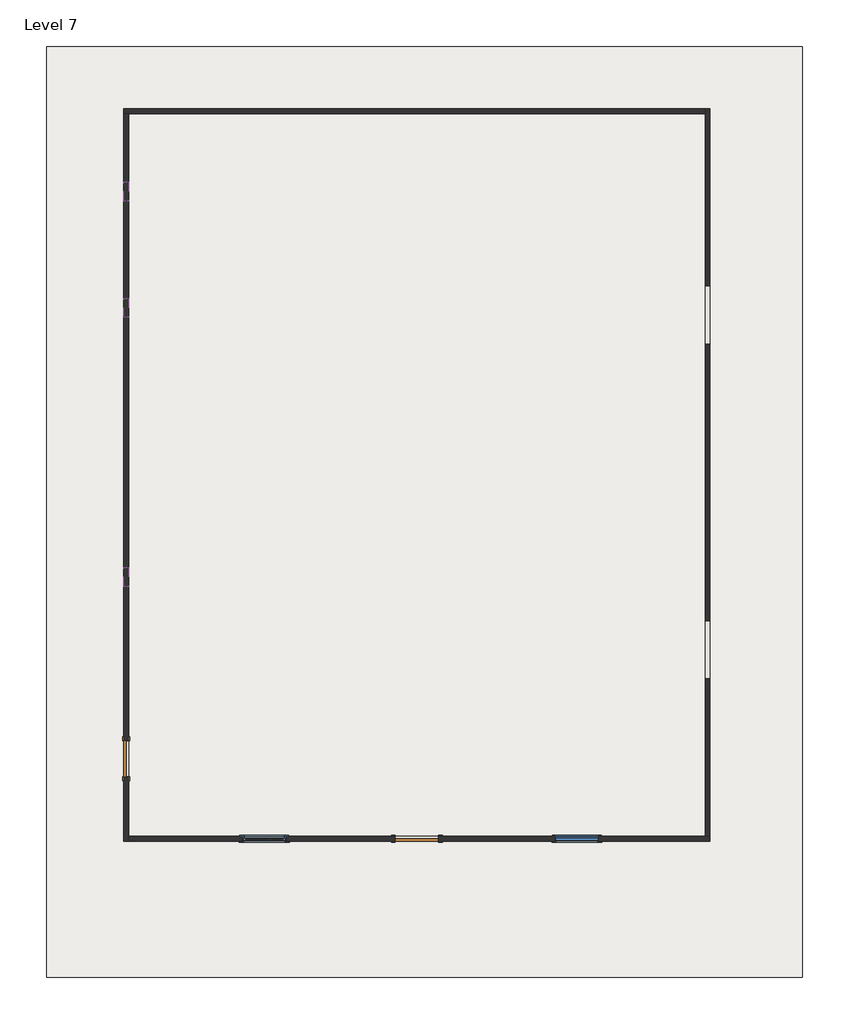
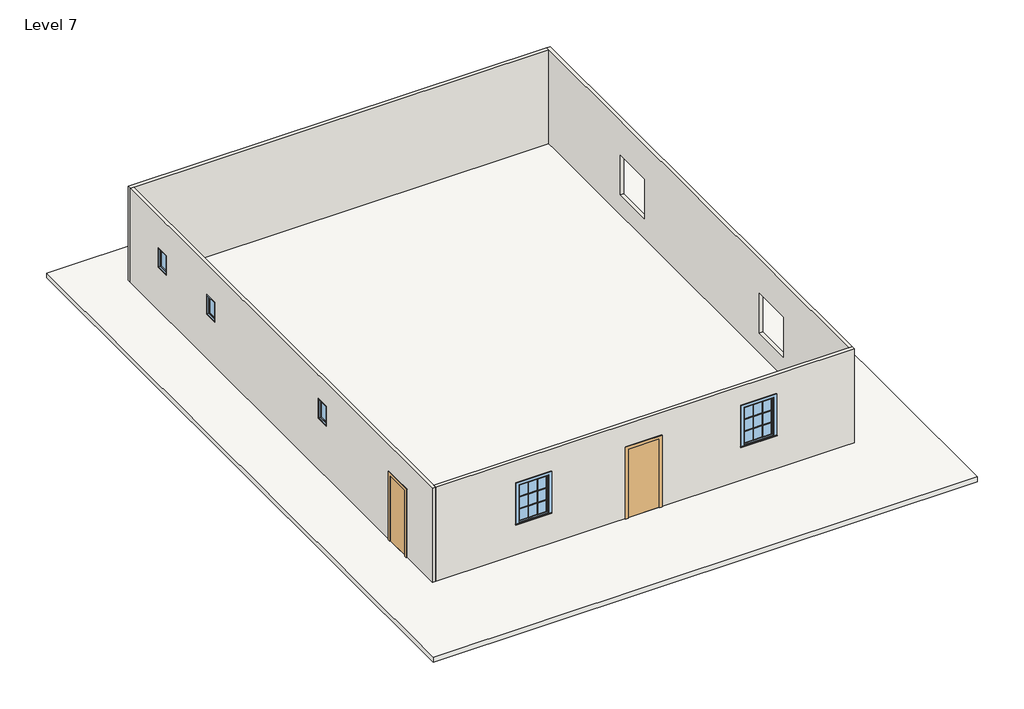
# One storey, incomplete: 5 windows, 4 walls, 2 doors, 1 roof.
"""IFC4 building model written with IfcOpenShell, lengths in millimetres."""

from ifc_helpers import new_model, si_unit, frame, origin, place, context, project, spatial, polyline, outline, extrude, faceted_brep, transform, mapped, element, save
from components import door_29583826, door_048588e9, window_ad8769eb, window_a112695e

model = new_model("IFC4")

# Units and contexts
model_context = context("Model", 3, world=origin())
ifc_project = project(units=[si_unit("LENGTHUNIT", "METRE", prefix="MILLI")], contexts=[model_context])

# Site, building, storey
site = spatial("IfcSite", under=ifc_project)
building = spatial("IfcBuilding", under=site)
storey = spatial("IfcBuildingStorey", under=building, Name="Level 7", Elevation=9601.2)

# Doors
placement = place(None, origin())
door_shape = door_29583826(model_context)
element("IfcDoor", 1, ObjectType="Single-Flush : 30\" x 80\"", at=placement, inside=storey, context=model_context, shape_type="MappedRepresentation", body=[
    mapped(door_shape, transform((1744.5168112, -314.4718204, 9753.6), x_axis=(0.0, 1.0, 0.0), y_axis=(-1.0, 0.0, 0.0), z_axis=(0.0, 0.0, 1.0))),
])
door_2_shape = door_048588e9(model_context)
element("IfcDoor", 2, ObjectType="Single-Flush : 36\" x 84\"", at=placement, inside=storey, context=model_context, shape_type="MappedRepresentation", body=[
    mapped(door_2_shape, transform((7840.5168112, -1990.8718204, 9753.6), x_axis=(-1.0, 0.0, 0.0), y_axis=(0.0, -1.0, 0.0), z_axis=(0.0, 0.0, 1.0))),
])

# Roof
element("IfcRoof", 3, ObjectType="6", at=placement, inside=storey, context=model_context, shape_type="SweptSolid", body=[
    extrude(outline(polyline([(74.1689082, 14608.7600271), (15923.7689082, 14608.7600271), (15923.7689082, -4898.4399729), (74.1689082, -4898.4399729), (74.1689082, 14608.7600271)])), frame((0.0, 0.0, 9601.2), z_axis=(0.0, 0.0, 1.0), x_axis=(1.0, 0.0, 0.0)), (0.0, 0.0, 1.0), 152.4),
])

# Walls
element("IfcWall", 4, ObjectType="Generic - 4\" Brick", at=placement, inside=storey, context=model_context, shape_type="Brep", body=[
    faceted_brep([(1693.7168112, 13198.3281796, 9601.2), (1795.3168112, 13198.3281796, 9601.2), (13885.7168112, 13198.3281796, 9601.2), (13885.7168112, 13198.3281796, 12649.2), (1795.3168112, 13198.3281796, 12649.2), (1693.7168112, 13198.3281796, 12649.2), (1693.7168112, 13299.9281796, 9601.2), (1693.7168112, 13299.9281796, 12649.2), (13885.7168112, 13299.9281796, 12649.2), (13885.7168112, 13299.9281796, 9601.2)], [[[0, 1, 2, 3, 4, 5]], [[6, 7, 8, 9]], [[2, 1, 0, 6, 9]], [[0, 5, 7, 6]], [[3, 2, 9, 8]], [[5, 4, 3, 8, 7]]]),
])
element("IfcWall", 5, ObjectType="Generic - 4\" Brick", at=placement, inside=storey, context=model_context, shape_type="Brep", body=[
    faceted_brep([(1795.3168112, -2041.6718204, 9601.2), (1795.3168112, -1940.0718204, 9601.2), (1795.3168112, 13198.3281796, 9601.2), (1795.3168112, 13198.3281796, 12649.2), (1795.3168112, -1940.0718204, 12649.2), (1795.3168112, -2041.6718204, 12649.2), (1795.3168112, -695.4718204, 9753.6), (1795.3168112, -695.4718204, 11785.6), (1795.3168112, 66.5281796, 11785.6), (1795.3168112, 66.5281796, 9753.6), (1795.3168112, 11369.5281796, 11689.2182753), (1795.3168112, 11775.9281796, 11689.2182753), (1795.3168112, 11775.9281796, 11079.6182753), (1795.3168112, 11369.5281796, 11079.6182753), (1795.3168112, 8931.1281796, 11725.7539428), (1795.3168112, 9337.5281796, 11725.7539428), (1795.3168112, 9337.5281796, 11116.1539428), (1795.3168112, 8931.1281796, 11116.1539428), (1795.3168112, 3292.3281796, 11939.4851545), (1795.3168112, 3698.7281796, 11939.4851545), (1795.3168112, 3698.7281796, 11329.8851545), (1795.3168112, 3292.3281796, 11329.8851545), (1693.7168112, -2041.6718204, 9601.2), (1693.7168112, -2041.6718204, 12649.2), (1693.7168112, 13198.3281796, 12649.2), (1693.7168112, 13198.3281796, 9601.2), (1693.7168112, -695.4718204, 9753.6), (1693.7168112, 66.5281796, 9753.6), (1693.7168112, 66.5281796, 11785.6), (1693.7168112, -695.4718204, 11785.6), (1693.7168112, 11369.5281796, 11689.2182753), (1693.7168112, 11369.5281796, 11079.6182753), (1693.7168112, 11775.9281796, 11079.6182753), (1693.7168112, 11775.9281796, 11689.2182753), (1693.7168112, 8931.1281796, 11725.7539428), (1693.7168112, 8931.1281796, 11116.1539428), (1693.7168112, 9337.5281796, 11116.1539428), (1693.7168112, 9337.5281796, 11725.7539428), (1693.7168112, 3292.3281796, 11939.4851545), (1693.7168112, 3292.3281796, 11329.8851545), (1693.7168112, 3698.7281796, 11329.8851545), (1693.7168112, 3698.7281796, 11939.4851545)], [[[0, 1, 2, 3, 4, 5], [6, 7, 8, 9], [10, 11, 12, 13], [14, 15, 16, 17], [18, 19, 20, 21]], [[22, 23, 24, 25], [26, 27, 28, 29], [30, 31, 32, 33], [34, 35, 36, 37], [38, 39, 40, 41]], [[2, 1, 0, 22, 25]], [[0, 5, 23, 22]], [[3, 2, 25, 24]], [[5, 4, 3, 24, 23]], [[27, 26, 6, 9]], [[28, 27, 9, 8]], [[29, 28, 8, 7]], [[26, 29, 7, 6]], [[31, 30, 10, 13]], [[32, 31, 13, 12]], [[33, 32, 12, 11]], [[30, 33, 11, 10]], [[35, 34, 14, 17]], [[36, 35, 17, 16]], [[37, 36, 16, 15]], [[34, 37, 15, 14]], [[39, 38, 18, 21]], [[40, 39, 21, 20]], [[41, 40, 20, 19]], [[38, 41, 19, 18]]]),
])
element("IfcWall", 6, ObjectType="Generic - 4\" Brick", at=placement, inside=storey, context=model_context, shape_type="Brep", body=[
    faceted_brep([(13987.3168112, -1940.0718204, 9601.2), (13885.7168112, -1940.0718204, 9601.2), (1795.3168112, -1940.0718204, 9601.2), (1795.3168112, -1940.0718204, 12649.2), (13885.7168112, -1940.0718204, 12649.2), (13987.3168112, -1940.0718204, 12649.2), (8297.7168112, -1940.0718204, 9753.6), (8297.7168112, -1940.0718204, 11887.2), (7383.3168112, -1940.0718204, 11887.2), (7383.3168112, -1940.0718204, 9753.6), (4182.9168112, -1940.0718204, 11907.6881646), (4182.9168112, -1940.0718204, 10688.4881646), (5097.3168112, -1940.0718204, 10688.4881646), (5097.3168112, -1940.0718204, 11907.6881646), (10736.1168112, -1940.0718204, 11999.2796438), (10736.1168112, -1940.0718204, 10780.0796438), (11650.5168112, -1940.0718204, 10780.0796438), (11650.5168112, -1940.0718204, 11999.2796438), (13987.3168112, -2041.6718204, 9601.2), (13987.3168112, -2041.6718204, 12649.2), (1795.3168112, -2041.6718204, 12649.2), (1795.3168112, -2041.6718204, 9601.2), (8297.7168112, -2041.6718204, 9753.6), (7383.3168112, -2041.6718204, 9753.6), (7383.3168112, -2041.6718204, 11887.2), (8297.7168112, -2041.6718204, 11887.2), (4182.9168112, -2041.6718204, 11907.6881646), (5097.3168112, -2041.6718204, 11907.6881646), (5097.3168112, -2041.6718204, 10688.4881646), (4182.9168112, -2041.6718204, 10688.4881646), (10736.1168112, -2041.6718204, 11999.2796438), (11650.5168112, -2041.6718204, 11999.2796438), (11650.5168112, -2041.6718204, 10780.0796438), (10736.1168112, -2041.6718204, 10780.0796438)], [[[0, 1, 2, 3, 4, 5], [6, 7, 8, 9], [10, 11, 12, 13], [14, 15, 16, 17]], [[18, 19, 20, 21], [22, 23, 24, 25], [26, 27, 28, 29], [30, 31, 32, 33]], [[2, 1, 0, 18, 21]], [[0, 5, 19, 18]], [[3, 2, 21, 20]], [[5, 4, 3, 20, 19]], [[23, 22, 6, 9]], [[24, 23, 9, 8]], [[25, 24, 8, 7]], [[22, 25, 7, 6]], [[11, 10, 26, 29]], [[12, 11, 29, 28]], [[13, 12, 28, 27]], [[10, 13, 27, 26]], [[15, 14, 30, 33]], [[16, 15, 33, 32]], [[17, 16, 32, 31]], [[14, 17, 31, 30]]]),
])
element("IfcWall", 7, ObjectType="Generic - 4\" Brick", at=placement, inside=storey, context=model_context, shape_type="Brep", body=[
    faceted_brep([(13885.7168112, 13299.9281796, 9601.2), (13885.7168112, 13198.3281796, 9601.2), (13885.7168112, -1940.0718204, 9601.2), (13885.7168112, -1940.0718204, 12649.2), (13885.7168112, 13198.3281796, 12649.2), (13885.7168112, 13299.9281796, 12649.2), (13885.7168112, 1361.9281796, 11582.4), (13885.7168112, 1361.9281796, 10363.2), (13885.7168112, 2581.1281796, 10363.2), (13885.7168112, 2581.1281796, 11582.4), (13885.7168112, 8372.3281796, 11582.4), (13885.7168112, 8372.3281796, 10363.2), (13885.7168112, 9591.5281796, 10363.2), (13885.7168112, 9591.5281796, 11582.4), (13987.3168112, 13299.9281796, 9601.2), (13987.3168112, 13299.9281796, 12649.2), (13987.3168112, -1940.0718204, 12649.2), (13987.3168112, -1940.0718204, 9601.2), (13987.3168112, 1361.9281796, 11582.4), (13987.3168112, 2581.1281796, 11582.4), (13987.3168112, 2581.1281796, 10363.2), (13987.3168112, 1361.9281796, 10363.2), (13987.3168112, 8372.3281796, 11582.4), (13987.3168112, 9591.5281796, 11582.4), (13987.3168112, 9591.5281796, 10363.2), (13987.3168112, 8372.3281796, 10363.2)], [[[0, 1, 2, 3, 4, 5], [6, 7, 8, 9], [10, 11, 12, 13]], [[14, 15, 16, 17], [18, 19, 20, 21], [22, 23, 24, 25]], [[2, 1, 0, 14, 17]], [[0, 5, 15, 14]], [[3, 2, 17, 16]], [[5, 4, 3, 16, 15]], [[7, 6, 18, 21]], [[8, 7, 21, 20]], [[9, 8, 20, 19]], [[6, 9, 19, 18]], [[11, 10, 22, 25]], [[12, 11, 25, 24]], [[13, 12, 24, 23]], [[10, 13, 23, 22]]]),
])

# Windows
window_shape = window_ad8769eb(model_context)
element("IfcWindow", 8, ObjectType="Casement 3x3 with Trim : 36\" x 48\"", at=placement, inside=storey, context=model_context, shape_type="MappedRepresentation", body=[
    mapped(window_shape, transform((4640.1168112, -1990.8718204, 9774.0881646), x_axis=(-1.0, 0.0, 0.0), y_axis=(0.0, -1.0, 0.0), z_axis=(0.0, 0.0, 1.0))),
])
element("IfcWindow", 9, ObjectType="Casement 3x3 with Trim : 36\" x 48\"", at=placement, inside=storey, context=model_context, shape_type="MappedRepresentation", body=[
    mapped(window_shape, transform((11193.3168112, -1990.8718204, 9865.6796438), x_axis=(-1.0, 0.0, 0.0), y_axis=(0.0, -1.0, 0.0), z_axis=(0.0, 0.0, 1.0))),
])
window_2_shape = window_a112695e(model_context)
element("IfcWindow", 10, ObjectType="Fixed : 16\" x 24\"", at=placement, inside=storey, context=model_context, shape_type="MappedRepresentation", body=[
    mapped(window_2_shape, transform((1744.5168112, 11534.6281796, 10165.2182753), x_axis=(0.0, -1.0, 0.0), y_axis=(1.0, 0.0, 0.0), z_axis=(0.0, 0.0, 1.0))),
])
element("IfcWindow", 11, ObjectType="Fixed : 16\" x 24\"", at=placement, inside=storey, context=model_context, shape_type="MappedRepresentation", body=[
    mapped(window_2_shape, transform((1744.5168112, 9096.2281796, 10201.7539428), x_axis=(0.0, -1.0, 0.0), y_axis=(1.0, 0.0, 0.0), z_axis=(0.0, 0.0, 1.0))),
])
element("IfcWindow", 12, ObjectType="Fixed : 16\" x 24\"", at=placement, inside=storey, context=model_context, shape_type="MappedRepresentation", body=[
    mapped(window_2_shape, transform((1744.5168112, 3457.4281796, 10415.4851545), x_axis=(0.0, -1.0, 0.0), y_axis=(1.0, 0.0, 0.0), z_axis=(0.0, 0.0, 1.0))),
])

save(model, "model.ifc")

# Revit data of these elements
# Type "Single-Flush : 30\" x 80\""
#   Type Mark = "5"
#   Construction Type Id = "MDOOR"
#   Assembly Code = "C1020"
#   Analytic Construction = "Metal"
#   Thickness = 0' - 2"
#   Heat Transfer Coefficient (U) = 0.651978 BTU/(h·ft²·°F)
#   Height = 6' - 8"
#   Trim Projection Ext = 0' - 1"
#   Trim Projection Int = 0' - 1"
#   Trim Width = 0' - 3"
#   Width = 2' - 6"
#   Define Thermal Properties by = 1
#   Door Material = Door - Panel
#   Frame Material = Door - Frame
#   Visual Light Transmittance = 0
#   Solar Heat Gain Coefficient = 0
#   Function = (empty or 0)
#   Wall Closure = (empty or 0)
# Type "Single-Flush : 36\" x 84\""
#   Type Mark = "1"
#   Construction Type Id = "MDOOR"
#   Assembly Code = "C1020"
#   Analytic Construction = "Metal"
#   Thickness = 0' - 2"
#   Heat Transfer Coefficient (U) = 0.651978 BTU/(h·ft²·°F)
#   Height = 7' - 0"
#   Trim Projection Ext = 0' - 1"
#   Trim Projection Int = 0' - 1"
#   Trim Width = 0' - 3"
#   Width = 3' - 0"
#   Define Thermal Properties by = 1
#   Door Material = Door - Panel
#   Frame Material = Door - Frame
#   Visual Light Transmittance = 0
#   Solar Heat Gain Coefficient = 0
#   Function = (empty or 0)
#   Wall Closure = (empty or 0)
# Type "6"
#   Assembly Code = "B1020"
#   Layers, outside or top first: 0' - 6" no material (function 1)
# Type "Generic - 4\" Brick"
#   Assembly Code = "B2010"
#   Layers, outside or top first: 0' - 4" "Brick, Common" (function 1)
# Type "Casement 3x3 with Trim : 36\" x 48\""
#   Type Mark = "10"
#   Construction Type Id = "GSP4R"
#   Assembly Code = "B2020100"
#   Analytic Construction = "1/8 in Pilkington single glazing"
#   Visual Light Transmittance = 0.9
#   Solar Heat Gain Coefficient = 0.78
#   Heat Transfer Coefficient (U) = 0.6496 BTU/(h·ft²·°F)
#   Height = 4' - 0"
#   Default Sill Height = 3' - 0"
#   Trim Projection - Ext. = 0' - 0 1/2"
#   Trim Projection - Int. = 0' - 0 3/4"
#   Trim Width - Exterior = 0' - 3 1/2"
#   Trim Width - Interior = 0' - 3 1/2"
#   Width = 3' - 0"
#   Window Inset = 0' - 0 3/4"
#   Define Thermal Properties by = 1
#   Glass Pane Material = Glass
#   Sash Material = Sash
#   Trim Exterior Material = Trim
#   Trim Interior Material = Trim
#   Wall Closure = (empty or 0)
# Type "Fixed : 16\" x 24\""
#   Type Mark = "4"
#   Construction Type Id = "GSP4R"
#   Assembly Code = "B2020100"
#   Analytic Construction = "1/8 in Pilkington single glazing"
#   Visual Light Transmittance = 0.9
#   Solar Heat Gain Coefficient = 0.78
#   Heat Transfer Coefficient (U) = 0.6496 BTU/(h·ft²·°F)
#   Height = 2' - 0"
#   Default Sill Height = 3' - 0"
#   Width = 1' - 4"
#   Window Inset = 0' - 0 3/4"
#   Define Thermal Properties by = 1
#   Glass Pane Material = Glass
#   Sash Material = Sash
#   Wall Closure = (empty or 0)
# Element 1 (IfcDoor, "Single-Flush : 30\" x 80\"")
#   Phase Created = New Construction
#   Materials on its faces: "Door - Frame", "Door - Panel"
# Element 2 (IfcDoor, "Single-Flush : 36\" x 84\"")
#   Phase Created = New Construction
#   Materials on its faces: "Door - Frame", "Door - Panel"
# Element 3 (IfcRoof, "6")
#   built-in parameter 1001705 = 32 (stored number, unit not read)
#   built-in parameter 1001710 = 33615
#   Phase Created = New Construction
#   Materials on its faces: "Default Roof"
# Elements 4, 5, 6, 7 (IfcWall, "Generic - 4\" Brick")
#   Top Offset = 0' - 0"
#   Base Offset = 0' - 0"
#   Unconnected Height = 10' - 0"
#   wall height = 10' - 0"
#   Phase Created = New Construction
#   Base Constraint = Level 7
#   Materials on its faces: "Brick, Common"
# Element 8 (IfcWindow, "Casement 3x3 with Trim : 36\" x 48\"")
#   Mark = "19"
#   Phase Created = New Construction
#   Materials on its faces: "Sash", "Glass", "Trim"
# Element 9 (IfcWindow, "Casement 3x3 with Trim : 36\" x 48\"")
#   Mark = "20"
#   Phase Created = New Construction
#   Materials on its faces: "Sash", "Glass", "Trim"
# Element 10 (IfcWindow, "Fixed : 16\" x 24\"")
#   Mark = "7"
#   Phase Created = New Construction
#   Materials on its faces: "Sash", "Glass"
# Element 11 (IfcWindow, "Fixed : 16\" x 24\"")
#   Mark = "8"
#   Phase Created = New Construction
#   Materials on its faces: "Sash", "Glass"
# Element 12 (IfcWindow, "Fixed : 16\" x 24\"")
#   Mark = "12"
#   Phase Created = New Construction
#   Materials on its faces: "Sash", "Glass"
# Materials
#   "Door - Panel": class "Wood", colour RGB 210 159 95, transparency 0
#   "Door - Frame": colour RGB 118 70 51, transparency 0
#   "Brick, Common": class "Masonry", colour RGB 170 98 104, transparency 0, Description = "Common brick", Cost = 0
#   "Glass": class "Glass", colour RGB 0 128 192, transparency 0.75, Description = "Soda Lime Glass", Cost = 0
#   "Sash": class "Wood", colour RGB 224 178 126, transparency 0
#   "Trim": class "Wood", colour RGB 224 178 126, transparency 0
#   "Default Roof": colour RGB 88 101 114, transparency 0
